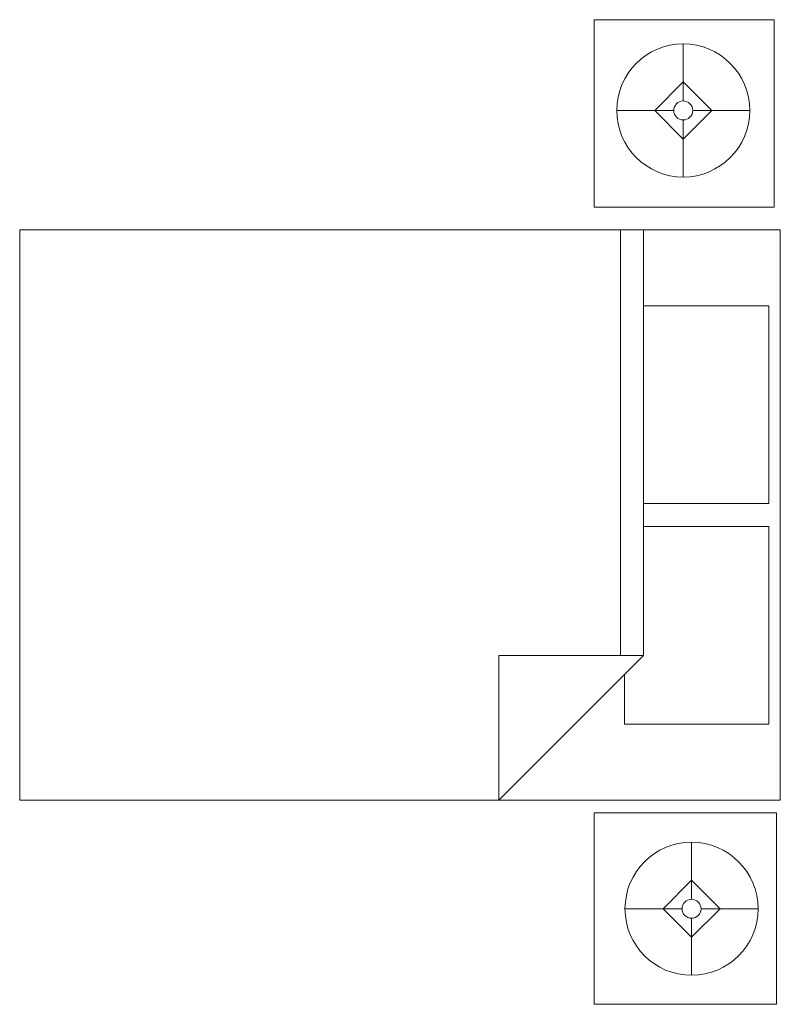
# Model space of a CAD drawing. Units: inches. Extents: x 50 to 2003, y -28 to 675.
# Tile 10 of 10: x 1923 to 2003, y 402 to 506. Entities that reach past the tile are written whole.
import ezdxf

# ---------------------------------------------------------------- set-up
doc = ezdxf.new("R2010")
doc.units = ezdxf.units.IN
doc.layers.add('A-FURN', color=8, linetype='Continuous', lineweight=18)
doc.layers.add('A-FURN-LITE', color=9, linetype='Continuous', lineweight=13)

# ---------------------------------------------------------------- blocks, each defined once
blk = doc.blocks.new('Bed - Queen')
for p, q in [((0, -80.00003), (0, 0)), ((0, 0), (59.99999, 0)), ((59.99999, 0), (59.99999, -80.00003)), ((7.99999, -1.2), (28.79998, -1.2)), ((7.99999, -14.4), (7.99999, -1.2)), ((28.79998, -1.2), (28.79998, -14.4)), ((31.19999, -1.2), (51.99999, -1.2)), ((31.19999, -14.4), (31.19999, -1.2)), ((51.99999, -1.2), (51.99999, -16.4)), ((0, -14.4), (44.8, -14.4)), ((59.99999, -29.6), (44.8, -14.4)), ((44.8, -14.4), (44.8, -29.6)), ((51.99999, -16.4), (46.79936, -16.4)), ((44.8, -16.8), (0, -16.8)), ((44.8, -29.6), (59.99999, -29.6)), ((59.99999, -80.00003), (0, -80.00003))]:
    blk.add_line(p, q)
blk = doc.blocks.new('Lamp - Table')
for p, q in [((0, 7), (0, 1)), ((0, 3), (-3, 0)), ((3, 0), (0, 3)), ((-1, 0), (-7, 0)), ((-3, 0), (0, -3)), ((0, -3), (3, 0)), ((1, 0), (7, 0)), ((0, -1), (0, -7))]:
    blk.add_line(p, q)
for radius in [7, 1]:
    blk.add_circle((0, 0), radius)
blk = doc.blocks.new('NIGHTSTAND-COMPACT')
blk.add_lwpolyline([(0, 19.73), (0, 0), (18.92, 0), (18.92, 19.73)], close=True)
blk = doc.blocks.new('NIGHTSTAND-STANDARD')
blk.add_lwpolyline([(0, 0), (0, 20.13), (19.19, 20.13), (19.19, 0)], close=True)

msp = doc.modelspace()

# ---------------------------------------------------------------- block references
at = {"layer": 'A-FURN'}
for name, p, rotation in [('NIGHTSTAND-COMPACT', (2002.5098, 505.9582), 180), ('Bed - Queen', (2003.1701, 483.8417), 270), ('NIGHTSTAND-STANDARD', (2002.7763, 422.488), 180)]:
    msp.add_blockref(name, p, dxfattribs=dict(at, rotation=rotation))
at = {"layer": 'A-FURN-LITE', "rotation": 270}
for p in [(1992.9616, 496.4038), (1993.8347, 412.406)]:
    msp.add_blockref('Lamp - Table', p, dxfattribs=at)

doc.saveas('drawing.dxf')
